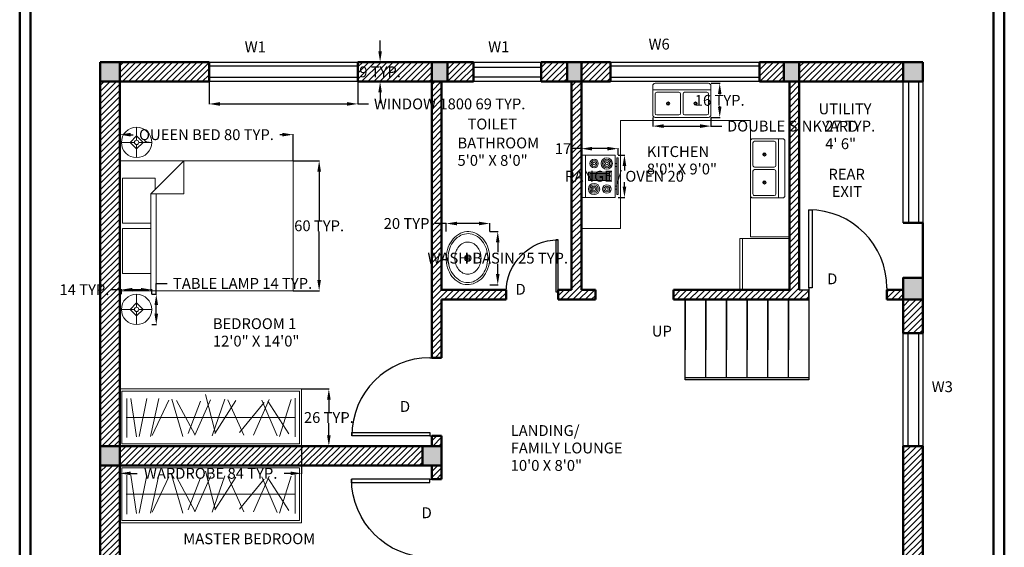
# Model space of a CAD drawing. Units: inches. Extents: x -25 to 429, y -18 to 847.
# Tile 2 of 3: x -25 to 429, y 226 to 470. Entities that reach past the tile are written whole.
import ezdxf

# ---------------------------------------------------------------- set-up
doc = ezdxf.new("R2010")
doc.units = ezdxf.units.IN
doc.header["$MEASUREMENT"] = 0
for name, color, linetype, lineweight in [('A-ANNO-DIMS', 2, 'Continuous', 18), ('A-ANNO-TEXT', 3, 'Continuous', 25), ('A-ANNO-TTLB', 7, 'Continuous', 50), ('A-AREA-IDEN', 7, 'Continuous', 25), ('A-DOOR', 4, 'Continuous', 25), ('A-FLOR-FIXT', 8, 'Continuous', 18), ('A-FLOR-STRS', 3, 'Continuous', 25), ('A-FURN', 8, 'Continuous', 18), ('A-GLAZ', 4, 'Continuous', 25), ('A-WALL', 7, 'Continuous', 50), ('A-WALL-FILL', 18, 'Continuous', 13), ('A-WALL-PATT', 252, 'Continuous', 13)]:
    doc.layers.add(name, color=color, linetype=linetype, lineweight=lineweight)
doc.styles.get("Standard").update_dxf_attribs({"font": 'arial.ttf'})
doc.dimstyles.get("Standard").update_dxf_attribs({"dimtxt": 5, "dimasz": 5, "dimexe": 0.18, "dimexo": 0.0625, "dimgap": 0.09, "dimtad": 0, "dimtih": 1, "dimtoh": 1, "dimdec": 1, "dimzin": 0, "dimdsep": 46, "dimlunit": 4, "dimtxsty": 'Standard', "dimcen": 0.09, "dimadec": 0, "dimazin": 0, "dimtfac": 1, "dimtdec": 1, "dimtofl": 0, "dimtmove": 0, "dimatfit": 3, "dimfxl": 1, "dimtolj": 1, "dimtzin": 0, "dimarcsym": 0})

# ---------------------------------------------------------------- blocks, each defined once
blk = doc.blocks.new('Bed - Queen')
for p, q in [((0, -80.00003), (0, 0)), ((0, 0), (59.99999, 0)), ((59.99999, 0), (59.99999, -80.00003)), ((7.99999, -1.2), (28.79998, -1.2)), ((7.99999, -14.4), (7.99999, -1.2)), ((28.79998, -1.2), (28.79998, -14.4)), ((31.19999, -1.2), (51.99999, -1.2)), ((31.19999, -14.4), (31.19999, -1.2)), ((51.99999, -1.2), (51.99999, -16.4)), ((0, -14.4), (44.8, -14.4)), ((44.8, -16.8), (0, -16.8)), ((59.99999, -29.6), (44.8, -14.4)), ((44.8, -14.4), (44.8, -29.6)), ((51.99999, -16.4), (46.79936, -16.4)), ((44.8, -29.6), (59.99999, -29.6)), ((59.99999, -80.00003), (0, -80.00003))]:
    blk.add_line(p, q)
blk = doc.blocks.new('Lamp - Table')
for p, q in [((0, 7), (0, 1)), ((-1, 0), (-7, 0)), ((0, 3), (-3, 0)), ((-3, 0), (0, -3)), ((3, 0), (0, 3)), ((0, -3), (3, 0)), ((1, 0), (7, 0)), ((0, -1), (0, -7))]:
    blk.add_line(p, q)
for radius in [7, 1]:
    blk.add_circle((0, 0), radius)
blk = doc.blocks.new('Range-Oven - 30 in top')
for p, q in [((0, -3), (30, -3)), ((12, -6), (18, -6)), ((13, -20), (13, -6)), ((14, -6), (14, -20)), ((15, -20), (15, -6)), ((16, -6), (16, -20)), ((17, -20), (17, -6)), ((18, -20), (12, -20)), ((6, -24), (6, -25)), ((8, -25), (8, -24)), ((22, -25), (22, -24)), ((24, -24), (24, -25))]:
    blk.add_line(p, q)
for points in [[(0, -24), (0, 0), (30, 0), (30, -24)], [(12, -21), (12, -5), (18, -5), (18, -21)], [(2, -26), (2, -25), (28, -25), (28, -26)]]:
    blk.add_lwpolyline(points, close=True)
for centre, radius in [((6, -9), 4), ((6, -9), 3), ((24, -9), 3), ((6, -9), 2), ((6, -9), 1), ((24, -9), 2), ((24, -9), 1), ((6, -18), 3), ((6, -18), 2), ((6, -18), 1), ((24, -18), 4), ((24, -18), 3), ((24, -18), 2), ((24, -18), 1)]:
    blk.add_circle(centre, radius)
blk = doc.blocks.new('Sink-double - 36 in top')
for p, q in [((-18, -4), (18, -4)), ((-0.75, -18.5), (-0.75, -6.5)), ((0.75, -6.5), (0.75, -18.5))]:
    blk.add_line(p, q)
for points in [[(-16.5, 0), (16.5, 0)], [(-18, -19.5), (-18, -1.5)], [(-15.5, -5.5), (-1.75, -5.5)], [(1.75, -5.5), (15.5, -5.5)], [(18, -1.5), (18, -19.5)], [(-16.5, -18.5), (-16.5, -6.5)], [(16.5, -6.5), (16.5, -18.5)], [(16.5, -21), (-16.5, -21)], [(-1.75, -19.5), (-15.5, -19.5)], [(15.5, -19.5), (1.75, -19.5)]]:
    blk.add_lwpolyline(points)
for centre, radius in [((-8.5, -12.5), 1), ((8.5, -12.5), 1), ((-8.5, -12.5), 0.5), ((8.5, -12.5), 0.5)]:
    blk.add_circle(centre, radius)
for centre, radius, start, end in [((-16.5, -1.5), 1.5, 90, 180), ((16.5, -1.5), 1.5, 0, 90), ((-15.5, -6.5), 1, 90, 180), ((-1.75, -6.5), 1, 0, 90), ((1.75, -6.5), 1, 90, 180), ((15.5, -6.5), 1, 0, 90), ((-16.5, -19.5), 1.5, 180, 270), ((-15.5, -18.5), 1, 180, 270), ((-1.75, -18.5), 1, 270, 0), ((1.75, -18.5), 1, 180, 270), ((15.5, -18.5), 1, 270, 0), ((16.5, -19.5), 1.5, 270, 0)]:
    blk.add_arc(centre, radius, start, end)
blk = doc.blocks.new('Sink - Oval top')
for p, q in [((-1, 0), (1, 0)), ((0, 1), (0, -1))]:
    blk.add_line(p, q)
for points in [[(-12.23, 0.39, 0.117634), (-11.46, -3.36, 0.104469), (-8.88, -6.8, 0.090016), (-5.08, -9.07, 0.08192), (-0.32, -10.02, 0.08192), (4.49, -9.38, 0.090016), (8.42, -7.36, 0.104469), (11.22, -4.09, 0.117634), (12.23, -0.39, 0.117634), (11.46, 3.36, 0.104469), (8.88, 6.8, 0.090016), (5.08, 9.07, 0.08192), (0.32, 10.02, 0.08192), (-4.49, 9.38, 0.090016), (-8.42, 7.36, 0.104469), (-11.22, 4.09, 0.117634)], [(-11.29, 0.16, 0.118622), (-10.52, -3.25, 0.104678), (-8.07, -6.36, 0.089562), (-4.54, -8.37, 0.081185), (-0.13, -9.15, 0.081185), (4.3, -8.49, 0.089562), (7.89, -6.58, 0.104678), (10.42, -3.55, 0.118622), (11.29, -0.16, 0.118622), (10.52, 3.25, 0.104678), (8.07, 6.36, 0.089562), (4.54, 8.37, 0.081185), (0.13, 9.15, 0.081185), (-4.3, 8.49, 0.089562), (-7.89, 6.58, 0.104678), (-10.42, 3.55, 0.118622)], [(-7.42, 0.08, 0.118283), (-6.91, -2.17, 0.104607), (-5.29, -4.21, 0.089718), (-2.97, -5.53, 0.081436), (-0.07, -6.04, 0.081436), (2.84, -5.59, 0.089718), (5.2, -4.33, 0.104607), (6.86, -2.32, 0.118283), (7.42, -0.08, 0.118283), (6.91, 2.17, 0.104607), (5.29, 4.21, 0.089718), (2.97, 5.53, 0.081436), (0.07, 6.04, 0.081436), (-2.84, 5.59, 0.089718), (-5.2, 4.33, 0.104607), (-6.86, 2.32, 0.118283)]]:
    blk.add_lwpolyline(points, format="xyb", close=True)
for radius in [1.5, 1]:
    blk.add_circle((0, 0), radius)
blk = doc.blocks.new('*U10')
for p, q in [((0, 0), (0, -6)), ((40, 0), (40, -6))]:
    blk.add_line(p, q)
blk.add_lwpolyline([(0, 0), (0, 40), (1.75, 40), (1.75, 0)], close=True)
blk.add_arc((0, 0), 40, 0, 90)
blk = doc.blocks.new('WIN-1800')
for points in [[(62.34, 449.99), (130.96, 449.99), (130.96, 440.99), (62.34, 440.99)], [(62.34, 448.22), (130.96, 448.22), (130.96, 442.88), (62.34, 442.88)]]:
    blk.add_lwpolyline(points, close=True)
blk = doc.blocks.new('WARDROBE')
for p, q in [((65.2, 279.42), (60.7, 296.77)), ((24.4, 294.9), (24.4, 276.98)), ((26.21, 294.93), (28.79, 277.19)), ((30.1, 277.36), (33.56, 294.94)), ((35.31, 277.4), (39.12, 294.91)), ((43.72, 294.1), (36.12, 277.87)), ((50.25, 277.42), (45.12, 294.59)), ((55.73, 278.26), (47.25, 294.05)), ((52.63, 278.85), (58.34, 293.66)), ((63.03, 294.35), (55.8, 277.95)), ((69.66, 294.66), (63.69, 277.76)), ((74.73, 293.93), (65.06, 278.84)), ((71.01, 294.33), (78.36, 277.98)), ((76.36, 279.22), (87.72, 293.08)), ((82.89, 277.99), (90.13, 294.39)), ((86.74, 294.18), (93.8, 277.71)), ((99.06, 278.61), (89.44, 293.73)), ((100.23, 294.49), (94.82, 277.41)), ((102.02, 277.19), (102.02, 295.11)), ((24.13, 286.15), (102.02, 286.15)), ((87.63, 286.15), (69.71, 286.15))]:
    blk.add_line(p, q)
for points in [[(21.13, 272.99), (105.02, 272.99), (105.02, 299.31), (21.13, 299.31)], [(22.13, 273.99), (104.02, 273.99), (104.02, 298.31), (22.13, 298.31)]]:
    blk.add_lwpolyline(points, close=True)
blk = doc.blocks.new('*D13')
at = {"layer": 'A-ANNO-DIMS', "color": 0, "lineweight": -2, "ltscale": 0.5, "transparency": 16777216}
for p, q in [((37.97, 342.96), (37.97, 347.96)), ((37.97, 347.96), (42.97, 347.96)), ((35.93, 342.96), (38.15, 342.96)), ((37.97, 333.96), (37.97, 337.96)), ((35.93, 328.96), (38.15, 328.96))]:
    blk.add_line(p, q, dxfattribs=at)
at = {"layer": 'A-ANNO-DIMS', "color": 0, "lineweight": 100, "ltscale": 0.5, "transparency": 16777216}
for points in [[(37.13, 337.96), (38.8, 337.96), (37.97, 342.96)], [(37.13, 333.96), (38.8, 333.96), (37.97, 328.96)]]:
    blk.add_solid(points, dxfattribs=at)
at = {"layer": 'Defpoints', "color": 0, "lineweight": 100, "ltscale": 0.5, "transparency": 16777216}
for p in [(35.87, 342.96), (37.97, 342.96), (35.87, 328.96)]:
    blk.add_point(p, dxfattribs=at)
at = {"layer": 'A-ANNO-DIMS', "color": 0, "ltscale": 0.5, "transparency": 16777216, "insert": (77.8, 347.96), "char_height": 5, "attachment_point": 5}
blk.add_mtext('\\A1;TABLE LAMP 14 TYP.', dxfattribs=at)
blk = doc.blocks.new('*D14')
at = {"layer": 'A-ANNO-DIMS', "color": 0, "lineweight": -2, "ltscale": 0.5, "transparency": 16777216}
for p, q in [((21.87, 345.06), (16.87, 345.06)), ((21.87, 343.02), (21.87, 345.24)), ((30.87, 345.06), (26.87, 345.06)), ((35.87, 343.02), (35.87, 345.24))]:
    blk.add_line(p, q, dxfattribs=at)
at = {"layer": 'A-ANNO-DIMS', "color": 0, "lineweight": 100, "ltscale": 0.5, "transparency": 16777216}
for points in [[(26.87, 345.89), (26.87, 344.23), (21.87, 345.06)], [(30.87, 345.89), (30.87, 344.23), (35.87, 345.06)]]:
    blk.add_solid(points, dxfattribs=at)
at = {"layer": 'Defpoints', "color": 0, "lineweight": 100, "ltscale": 0.5, "transparency": 16777216}
for p in [(21.87, 345.06), (21.87, 342.96), (35.87, 342.96)]:
    blk.add_point(p, dxfattribs=at)
at = {"layer": 'A-ANNO-DIMS', "color": 0, "ltscale": 0.5, "transparency": 16777216, "insert": (4.84, 345.06), "char_height": 5, "attachment_point": 5}
blk.add_mtext('\\A1;14 TYP.', dxfattribs=at)
blk = doc.blocks.new('*D15')
at = {"layer": 'A-ANNO-DIMS', "color": 0, "lineweight": -2, "ltscale": 0.5, "transparency": 16777216}
for p, q in [((191.92, 371.9), (195.72, 371.9)), ((195.54, 366.9), (195.54, 362.3)), ((195.54, 352.35), (195.54, 356.95)), ((191.92, 347.35), (195.72, 347.35))]:
    blk.add_line(p, q, dxfattribs=at)
at = {"layer": 'A-ANNO-DIMS', "color": 0, "lineweight": 100, "ltscale": 0.5, "transparency": 16777216}
for points in [[(194.7, 366.9), (196.37, 366.9), (195.54, 371.9)], [(194.7, 352.35), (196.37, 352.35), (195.54, 347.35)]]:
    blk.add_solid(points, dxfattribs=at)
at = {"layer": 'Defpoints', "color": 0, "lineweight": 100, "ltscale": 0.5, "transparency": 16777216}
for p in [(191.85, 371.9), (195.54, 371.9), (191.85, 347.35)]:
    blk.add_point(p, dxfattribs=at)
at = {"layer": 'A-ANNO-DIMS', "color": 0, "ltscale": 0.5, "transparency": 16777216, "insert": (195.54, 359.62), "char_height": 5, "attachment_point": 5}
blk.add_mtext('\\A1;WASH BASIN 25 TYP.', dxfattribs=at)
blk = doc.blocks.new('*D16')
at = {"layer": 'A-ANNO-DIMS', "color": 0, "lineweight": -2, "ltscale": 0.5, "transparency": 16777216}
for p, q in [((171.72, 375.58), (166.72, 375.58)), ((171.72, 371.96), (171.72, 375.76)), ((186.85, 375.58), (176.72, 375.58)), ((191.85, 371.96), (191.85, 375.76))]:
    blk.add_line(p, q, dxfattribs=at)
at = {"layer": 'A-ANNO-DIMS', "color": 0, "lineweight": 100, "ltscale": 0.5, "transparency": 16777216}
for points in [[(176.72, 376.41), (176.72, 374.75), (171.72, 375.58)], [(186.85, 376.41), (186.85, 374.75), (191.85, 375.58)]]:
    blk.add_solid(points, dxfattribs=at)
at = {"layer": 'Defpoints', "color": 0, "lineweight": 100, "ltscale": 0.5, "transparency": 16777216}
for p in [(171.72, 375.58), (171.72, 371.9), (191.85, 371.9)]:
    blk.add_point(p, dxfattribs=at)
at = {"layer": 'A-ANNO-DIMS', "color": 0, "ltscale": 0.5, "transparency": 16777216, "insert": (154.41, 375.58), "char_height": 5, "attachment_point": 5}
blk.add_mtext('\\A1;20 TYP.', dxfattribs=at)
blk = doc.blocks.new('*D17')
at = {"layer": 'A-ANNO-DIMS', "color": 0, "lineweight": -2, "ltscale": 0.5, "transparency": 16777216}
for p, q in [((21.13, 404.6), (21.13, 416.71)), ((26.13, 416.53), (27.33, 416.53)), ((96.13, 416.53), (94.92, 416.53)), ((101.13, 404.6), (101.13, 416.71))]:
    blk.add_line(p, q, dxfattribs=at)
at = {"layer": 'A-ANNO-DIMS', "color": 0, "lineweight": 100, "ltscale": 0.5, "transparency": 16777216}
for points in [[(26.13, 417.37), (26.13, 415.7), (21.13, 416.53)], [(96.13, 417.37), (96.13, 415.7), (101.13, 416.53)]]:
    blk.add_solid(points, dxfattribs=at)
at = {"layer": 'Defpoints', "color": 0, "lineweight": 100, "ltscale": 0.5, "transparency": 16777216}
for p in [(21.13, 416.53), (21.13, 404.53), (101.13, 404.53)]:
    blk.add_point(p, dxfattribs=at)
at = {"layer": 'A-ANNO-DIMS', "color": 0, "ltscale": 0.5, "transparency": 16777216, "insert": (61.13, 416.53), "char_height": 5, "attachment_point": 5}
blk.add_mtext('\\A1;QUEEN BED 80 TYP.', dxfattribs=at)
blk = doc.blocks.new('*D18')
at = {"layer": 'A-ANNO-DIMS', "color": 0, "lineweight": -2, "ltscale": 0.5, "transparency": 16777216}
for p, q in [((101.19, 404.53), (113.31, 404.53)), ((113.13, 399.53), (113.13, 377.18)), ((113.13, 349.53), (113.13, 371.89)), ((101.19, 344.53), (113.31, 344.53))]:
    blk.add_line(p, q, dxfattribs=at)
at = {"layer": 'A-ANNO-DIMS', "color": 0, "lineweight": 100, "ltscale": 0.5, "transparency": 16777216}
for points in [[(112.29, 399.53), (113.96, 399.53), (113.13, 404.53)], [(112.29, 349.53), (113.96, 349.53), (113.13, 344.53)]]:
    blk.add_solid(points, dxfattribs=at)
at = {"layer": 'Defpoints', "color": 0, "lineweight": 100, "ltscale": 0.5, "transparency": 16777216}
for p in [(101.13, 404.53), (113.13, 404.53), (101.13, 344.53)]:
    blk.add_point(p, dxfattribs=at)
at = {"layer": 'A-ANNO-DIMS', "color": 0, "ltscale": 0.5, "transparency": 16777216, "insert": (113.13, 374.53), "char_height": 5, "attachment_point": 5}
blk.add_mtext('\\A1;60 TYP.', dxfattribs=at)
blk = doc.blocks.new('*D27')
at = {"layer": 'A-ANNO-DIMS', "color": 0, "lineweight": -2, "ltscale": 0.5, "transparency": 16777216}
for p, q in [((267.02, 424.45), (267.02, 420.3)), ((293.92, 424.45), (293.92, 420.3)), ((272.02, 420.48), (288.92, 420.48)), ((293.92, 420.48), (298.92, 420.48))]:
    blk.add_line(p, q, dxfattribs=at)
at = {"layer": 'A-ANNO-DIMS', "color": 0, "lineweight": 100, "ltscale": 0.5, "transparency": 16777216}
for points in [[(272.02, 421.31), (272.02, 419.65), (267.02, 420.48)], [(288.92, 421.31), (288.92, 419.65), (293.92, 420.48)]]:
    blk.add_solid(points, dxfattribs=at)
at = {"layer": 'Defpoints', "color": 0, "lineweight": 100, "ltscale": 0.5, "transparency": 16777216}
for p in [(267.02, 424.51), (293.92, 424.51), (293.92, 420.48)]:
    blk.add_point(p, dxfattribs=at)
at = {"layer": 'A-ANNO-DIMS', "color": 0, "ltscale": 0.5, "transparency": 16777216, "insert": (335.5, 420.48), "char_height": 5, "attachment_point": 5}
blk.add_mtext('\\A1;DOUBLE SINK 27 TYP.', dxfattribs=at)
blk = doc.blocks.new('*D28')
at = {"layer": 'A-ANNO-DIMS', "color": 0, "lineweight": -2, "ltscale": 0.5, "transparency": 16777216}
for p, q in [((293.98, 440.21), (298.13, 440.21)), ((297.95, 435.21), (297.95, 435)), ((297.95, 429.51), (297.95, 429.72)), ((293.98, 424.51), (298.13, 424.51))]:
    blk.add_line(p, q, dxfattribs=at)
at = {"layer": 'A-ANNO-DIMS', "color": 0, "lineweight": 100, "ltscale": 0.5, "transparency": 16777216}
for points in [[(297.12, 435.21), (298.78, 435.21), (297.95, 440.21)], [(297.12, 429.51), (298.78, 429.51), (297.95, 424.51)]]:
    blk.add_solid(points, dxfattribs=at)
at = {"layer": 'Defpoints', "color": 0, "lineweight": 100, "ltscale": 0.5, "transparency": 16777216}
for p in [(293.92, 440.21), (297.95, 440.21), (293.92, 424.51)]:
    blk.add_point(p, dxfattribs=at)
at = {"layer": 'A-ANNO-DIMS', "color": 0, "ltscale": 0.5, "transparency": 16777216, "insert": (297.95, 432.36), "char_height": 5, "attachment_point": 5}
blk.add_mtext('\\A1;16 TYP.', dxfattribs=at)
blk = doc.blocks.new('*D29')
at = {"layer": 'A-ANNO-DIMS', "color": 0, "lineweight": -2, "ltscale": 0.5, "transparency": 16777216}
for p, q in [((62.34, 440.93), (62.34, 430.52)), ((130.96, 440.93), (130.96, 430.52)), ((67.34, 430.7), (125.96, 430.7)), ((130.96, 430.7), (135.96, 430.7))]:
    blk.add_line(p, q, dxfattribs=at)
at = {"layer": 'A-ANNO-DIMS', "color": 0, "lineweight": 100, "ltscale": 0.5, "transparency": 16777216}
for points in [[(67.34, 431.53), (67.34, 429.86), (62.34, 430.7)], [(125.96, 431.53), (125.96, 429.86), (130.96, 430.7)]]:
    blk.add_solid(points, dxfattribs=at)
at = {"layer": 'Defpoints', "color": 0, "lineweight": 100, "ltscale": 0.5, "transparency": 16777216}
for p in [(62.34, 440.99), (130.96, 440.99), (130.96, 430.7)]:
    blk.add_point(p, dxfattribs=at)
at = {"layer": 'A-ANNO-DIMS', "color": 0, "ltscale": 0.5, "transparency": 16777216, "insert": (173.35, 430.7), "char_height": 5, "attachment_point": 5}
blk.add_mtext('\\A1;WINDOW 1800 69 TYP.', dxfattribs=at)
blk = doc.blocks.new('*D30')
at = {"layer": 'A-ANNO-DIMS', "color": 0, "lineweight": -2, "ltscale": 0.5, "transparency": 16777216}
for p, q in [((141.25, 454.99), (141.25, 459.99)), ((131.02, 449.99), (141.43, 449.99)), ((131.02, 440.99), (141.43, 440.99)), ((141.25, 435.99), (141.25, 430.99))]:
    blk.add_line(p, q, dxfattribs=at)
at = {"layer": 'A-ANNO-DIMS', "color": 0, "lineweight": 100, "ltscale": 0.5, "transparency": 16777216}
for points in [[(140.42, 454.99), (142.09, 454.99), (141.25, 449.99)], [(140.42, 435.99), (142.09, 435.99), (141.25, 440.99)]]:
    blk.add_solid(points, dxfattribs=at)
at = {"layer": 'Defpoints', "color": 0, "lineweight": 100, "ltscale": 0.5, "transparency": 16777216}
for p in [(130.96, 449.99), (141.25, 449.99), (130.96, 440.99)]:
    blk.add_point(p, dxfattribs=at)
at = {"layer": 'A-ANNO-DIMS', "color": 0, "ltscale": 0.5, "transparency": 16777216, "insert": (141.25, 445.49), "char_height": 5, "attachment_point": 5}
blk.add_mtext('\\A1;9 TYP.', dxfattribs=at)
blk = doc.blocks.new('*D31')
at = {"layer": 'A-ANNO-DIMS', "color": 0, "lineweight": -2, "ltscale": 0.5, "transparency": 16777216}
for p, q in [((21.13, 272.93), (21.13, 260.23)), ((105.02, 272.93), (105.02, 260.23)), ((26.13, 260.41), (29.17, 260.41)), ((100.02, 260.41), (96.97, 260.41))]:
    blk.add_line(p, q, dxfattribs=at)
at = {"layer": 'A-ANNO-DIMS', "color": 0, "lineweight": 100, "ltscale": 0.5, "transparency": 16777216}
for points in [[(26.13, 261.24), (26.13, 259.57), (21.13, 260.41)], [(100.02, 261.24), (100.02, 259.57), (105.02, 260.41)]]:
    blk.add_solid(points, dxfattribs=at)
at = {"layer": 'Defpoints', "color": 0, "lineweight": 100, "ltscale": 0.5, "transparency": 16777216}
for p in [(21.13, 272.99), (105.02, 272.99), (105.02, 260.41)]:
    blk.add_point(p, dxfattribs=at)
at = {"layer": 'A-ANNO-DIMS', "color": 0, "ltscale": 0.5, "transparency": 16777216, "insert": (63.07, 260.41), "char_height": 5, "attachment_point": 5}
blk.add_mtext('\\A1;WARDROBE 84 TYP.', dxfattribs=at)
blk = doc.blocks.new('*D32')
at = {"layer": 'A-ANNO-DIMS', "color": 0, "lineweight": -2, "ltscale": 0.5, "transparency": 16777216}
for p, q in [((105.08, 299.31), (117.78, 299.31)), ((117.6, 294.31), (117.6, 288.79)), ((117.6, 277.99), (117.6, 283.51)), ((105.08, 272.99), (117.78, 272.99))]:
    blk.add_line(p, q, dxfattribs=at)
at = {"layer": 'A-ANNO-DIMS', "color": 0, "lineweight": 100, "ltscale": 0.5, "transparency": 16777216}
for points in [[(116.77, 294.31), (118.44, 294.31), (117.6, 299.31)], [(116.77, 277.99), (118.44, 277.99), (117.6, 272.99)]]:
    blk.add_solid(points, dxfattribs=at)
at = {"layer": 'Defpoints', "color": 0, "lineweight": 100, "ltscale": 0.5, "transparency": 16777216}
for p in [(105.02, 299.31), (117.6, 299.31), (105.02, 272.99)]:
    blk.add_point(p, dxfattribs=at)
at = {"layer": 'A-ANNO-DIMS', "color": 0, "ltscale": 0.5, "transparency": 16777216, "insert": (117.6, 286.15), "char_height": 5, "attachment_point": 5}
blk.add_mtext('\\A1;26 TYP.', dxfattribs=at)
blk = doc.blocks.new('*D33')
at = {"layer": 'A-ANNO-DIMS', "color": 0, "lineweight": -2, "ltscale": 0.5, "transparency": 16777216}
for p, q in [((251.13, 407.15), (254.18, 407.15)), ((254, 402.15), (254, 400.04)), ((254, 392.57), (254, 394.68)), ((251.13, 387.57), (254.18, 387.57))]:
    blk.add_line(p, q, dxfattribs=at)
at = {"layer": 'A-ANNO-DIMS', "color": 0, "lineweight": 100, "ltscale": 0.5, "transparency": 16777216}
for points in [[(253.17, 402.15), (254.84, 402.15), (254, 407.15)], [(253.17, 392.57), (254.84, 392.57), (254, 387.57)]]:
    blk.add_solid(points, dxfattribs=at)
at = {"layer": 'Defpoints', "color": 0, "lineweight": 100, "ltscale": 0.5, "transparency": 16777216}
for p in [(251.07, 407.15), (254, 407.15), (251.07, 387.57)]:
    blk.add_point(p, dxfattribs=at)
at = {"layer": 'A-ANNO-DIMS', "color": 0, "ltscale": 0.5, "transparency": 16777216, "insert": (254, 397.36), "char_height": 5, "attachment_point": 5}
blk.add_mtext('\\A1;RANGE / OVEN 20', dxfattribs=at)
blk = doc.blocks.new('*D34')
at = {"layer": 'A-ANNO-DIMS', "color": 0, "lineweight": -2, "ltscale": 0.5, "transparency": 16777216}
for p, q in [((234.1, 410.08), (229.1, 410.08)), ((234.1, 407.21), (234.1, 410.26)), ((246.07, 410.08), (239.1, 410.08)), ((251.07, 407.21), (251.07, 410.26))]:
    blk.add_line(p, q, dxfattribs=at)
at = {"layer": 'A-ANNO-DIMS', "color": 0, "lineweight": 100, "ltscale": 0.5, "transparency": 16777216}
for points in [[(239.1, 410.92), (239.1, 409.25), (234.1, 410.08)], [(246.07, 410.92), (246.07, 409.25), (251.07, 410.08)]]:
    blk.add_solid(points, dxfattribs=at)
at = {"layer": 'Defpoints', "color": 0, "lineweight": 100, "ltscale": 0.5, "transparency": 16777216}
for p in [(234.1, 410.08), (234.1, 407.15), (251.07, 407.15)]:
    blk.add_point(p, dxfattribs=at)
at = {"layer": 'A-ANNO-DIMS', "color": 0, "ltscale": 0.5, "transparency": 16777216, "insert": (225.67, 410.08), "char_height": 5, "attachment_point": 5}
blk.add_mtext('\\A1;17', dxfattribs=at)

msp = doc.modelspace()

# ---------------------------------------------------------------- hatches: boundary and pattern name
at = {"layer": 'A-WALL-FILL'}
h = msp.add_hatch(color=256, dxfattribs=at)
h.dxf.hatch_style = 1
h.paths.add_polyline_path([(169.63, 272.99), (160.88, 272.99), (160.88, 263.99), (169.63, 263.99)])
h.paths.add_polyline_path([(21.13, 95.99), (12.13, 95.99), (12.13, 86.99), (21.13, 86.99)])
h.paths.add_polyline_path([(21.13, 272.99), (12.13, 272.99), (12.13, 263.99), (21.13, 263.99)])
h.paths.add_polyline_path([(391.63, 350.55), (382.63, 350.55), (382.63, 340.49), (391.63, 340.49)])
h.paths.add_polyline_path([(391.63, 71.99), (382.63, 71.99), (382.63, 62.99), (391.63, 62.99)])
h.paths.add_polyline_path([(391.63, 220.21), (382.63, 220.21), (382.63, 208.25), (391.63, 208.25)])
h.paths.add_polyline_path([(334.63, 449.99), (327.59, 449.99), (327.59, 440.99), (334.63, 440.99)])
h.paths.add_polyline_path([(391.63, 449.99), (382.63, 449.99), (382.63, 440.99), (391.63, 440.99)])
h.paths.add_polyline_path([(234.13, 449.99), (227.53, 449.99), (227.53, 440.99), (234.13, 440.99)])
h.paths.add_polyline_path([(172.34, 449.99), (165.13, 449.99), (165.13, 440.99), (172.34, 440.99)])
h.paths.add_polyline_path([(21.13, 449.99), (12.13, 449.99), (12.13, 440.99), (21.13, 440.99)])
at = {"layer": 'A-WALL-PATT'}
h = msp.add_hatch(dxfattribs=at)
h.set_pattern_fill('ANSI31', color=256, scale=16)
h.paths.add_polyline_path([(160.88, 272.99), (21.13, 272.99), (21.13, 263.99), (105.02, 263.99), (160.88, 263.99)])
h.paths.add_polyline_path([(169.63, 340.49), (199.38, 340.49), (199.38, 344.99), (169.63, 344.99), (169.63, 440.99), (165.13, 440.99), (165.13, 313.72), (169.63, 313.72)])
h.paths.add_polyline_path([(21.13, 440.99), (12.13, 440.99), (12.13, 272.99), (21.13, 272.99), (21.13, 299.31)])
h.paths.add_polyline_path([(62.34, 449.99), (21.13, 449.99), (21.13, 440.99), (62.34, 440.99)])
h.paths.add_polyline_path([(165.13, 449.99), (130.96, 449.99), (130.96, 440.99), (165.13, 440.99)])
h.paths.add_polyline_path([(184.34, 449.99), (172.34, 449.99), (172.34, 440.99), (184.34, 440.99)])
h.paths.add_polyline_path([(227.53, 449.99), (215.51, 449.99), (215.51, 440.99), (227.53, 440.99)])
h.paths.add_polyline_path([(247.61, 449.99), (234.13, 449.99), (234.13, 440.99), (247.61, 440.99)])
h.paths.add_polyline_path([(327.59, 449.99), (316.24, 449.99), (316.24, 440.99), (327.59, 440.99)])
h.paths.add_polyline_path([(234.1, 407.15), (234.12, 440.99), (229.63, 440.99), (229.63, 344.99), (223.38, 344.99), (223.38, 340.49), (240.63, 340.49), (240.63, 344.99), (234.13, 344.99), (234.13, 387.57), (234.1, 387.57)])
h.paths.add_polyline_path([(334.63, 440.99), (330.13, 440.99), (330.13, 344.99), (276.63, 344.99), (276.63, 340.49), (339.1, 340.49), (339.1, 344.99), (334.63, 344.99)])
h.paths.add_polyline_path([(382.63, 449.99), (334.63, 449.99), (334.63, 440.99), (382.63, 440.99)])
h.paths.add_polyline_path([(382.63, 344.99), (375.1, 344.99), (375.1, 340.49), (382.63, 340.49)])
h.paths.add_polyline_path([(391.63, 340.49), (382.63, 340.49), (382.63, 325.05), (391.63, 325.05)])
h.paths.add_polyline_path([(391.63, 273.01), (382.63, 273.01), (382.63, 220.21), (391.63, 220.21)])
h.paths.add_polyline_path([(391.63, 208.25), (382.63, 208.25), (382.63, 71.99), (391.63, 71.99)])
h.paths.add_polyline_path([(382.63, 71.99), (330.34, 71.99), (330.34, 62.99), (382.63, 62.99)])
h.paths.add_polyline_path([(262.4, 71.99), (235.63, 71.99), (235.63, 208.49), (224.79, 208.49), (224.79, 203.99), (231.13, 203.99), (231.13, 95.99), (169.63, 95.99), (169.63, 203.99), (200.79, 203.99), (200.79, 208.49), (169.63, 208.49), (169.63, 221.76), (165.13, 221.76), (165.13, 95.99), (154.17, 95.99), (154.17, 86.99), (231.13, 86.99), (231.13, 62.99), (262.4, 62.99)])
h.paths.add_polyline_path([(48.08, 95.99), (21.13, 95.99), (21.13, 86.99), (48.08, 86.99)])
h.paths.add_polyline_path([(21.13, 263.99), (12.13, 263.99), (12.13, 95.99), (21.13, 95.99)])
h.paths.add_polyline_path([(169.63, 263.99), (165.13, 263.99), (165.13, 257.76), (169.63, 257.76)])
h.paths.add_polyline_path([(169.63, 277.72), (165.13, 277.72), (165.13, 272.99), (169.63, 272.99)])

# ---------------------------------------------------------------- linework, layer by layer
at = {"layer": 'A-ANNO-TTLB', "ltscale": 0.5}
for points in [[(-25.05, 846.91), (429.28, 846.91), (429.28, -17.53), (-25.05, -17.53)], [(-20.05, 841.91), (424.28, 841.91), (424.28, -12.53), (-20.05, -12.53)]]:
    msp.add_lwpolyline(points, close=True, dxfattribs=at)
at = {"layer": 'A-FLOR-FIXT'}
for p, q in [((252.13, 373.32), (252.13, 422.99)), ((252.13, 422.99), (312.13, 422.99)), ((312.13, 422.99), (312.13, 369.49)), ((234.13, 373.32), (252.13, 373.32)), ((308.45, 368.71), (308.41, 345.02)), ((312.13, 369.49), (330.13, 369.49)), ((312.13, 345.02), (312.13, 344.99))]:
    msp.add_line(p, q, dxfattribs=at)
msp.add_lwpolyline([(330.13, 344.99), (307.3, 345.03), (307.3, 368.71), (330.13, 368.67)], close=True, dxfattribs=at)
at = {"layer": 'A-FLOR-STRS'}
for p, q in [((334.63, 344.99), (339.1, 344.99)), ((339.1, 340.49), (339.1, 344.99)), ((281.95, 303.49), (281.95, 340.49)), ((281.95, 340.49), (281.95, 317.33)), ((291.49, 304.49), (291.49, 340.49)), ((291.49, 340.49), (291.49, 317.33)), ((301.02, 304.49), (301.02, 340.49)), ((301.02, 340.49), (301.02, 317.33)), ((310.56, 304.49), (310.56, 340.49)), ((310.56, 340.49), (310.56, 317.33)), ((320.1, 304.49), (320.1, 340.49)), ((320.1, 340.49), (320.1, 317.33)), ((329.63, 304.49), (329.63, 340.49)), ((329.63, 340.49), (329.63, 317.33)), ((339.1, 340.49), (339.1, 303.49)), ((339.1, 304.49), (281.95, 304.49)), ((339.1, 303.49), (281.95, 303.49))]:
    msp.add_line(p, q, dxfattribs=at)
at = {"layer": 'A-GLAZ'}
for points in [[(184.34, 449.99), (215.51, 449.99), (215.51, 440.99), (184.34, 440.99)], [(184.34, 447.66), (215.51, 447.66), (215.51, 443.03), (184.34, 443.03)], [(382.63, 440.99), (391.63, 440.99), (391.63, 375.94), (382.63, 375.94)], [(385.24, 440.99), (389.64, 440.99), (389.64, 375.94), (385.24, 375.94)], [(382.63, 325.05), (391.63, 325.05), (391.63, 273.01), (382.63, 273.01)], [(384.98, 325.05), (389.63, 325.05), (389.63, 273.01), (384.98, 273.01)]]:
    msp.add_lwpolyline(points, close=True, dxfattribs=at)
at = {"layer": 'A-WALL'}
for p, q in [((12.13, 449.99), (62.34, 449.99)), ((12.13, 449.99), (12.13, 86.99)), ((21.13, 449.99), (21.13, 86.99)), ((62.34, 449.99), (62.34, 440.99)), ((130.96, 449.99), (130.96, 440.99)), ((130.96, 449.99), (184.34, 449.99)), ((165.13, 449.99), (165.13, 313.72)), ((184.34, 440.99), (184.34, 449.99)), ((215.51, 440.99), (215.51, 449.99)), ((215.51, 449.99), (247.61, 449.99)), ((234.13, 449.99), (234.13, 344.99)), ((247.61, 440.99), (247.61, 449.99)), ((316.24, 440.99), (316.24, 449.99)), ((316.24, 449.99), (391.63, 449.99)), ((334.63, 449.99), (334.63, 344.99)), ((382.63, 449.99), (382.63, 440.99)), ((391.63, 449.99), (391.63, 440.99)), ((12.13, 440.99), (62.34, 440.99)), ((130.96, 440.99), (165.13, 440.99)), ((169.63, 440.99), (169.63, 344.99)), ((169.63, 440.99), (184.34, 440.99)), ((215.51, 440.99), (229.63, 440.99)), ((229.63, 440.99), (229.63, 344.99)), ((234.13, 440.99), (247.61, 440.99)), ((316.24, 440.99), (391.63, 440.99)), ((330.13, 440.99), (330.13, 344.99)), ((382.63, 375.94), (391.63, 375.94)), ((382.63, 350.55), (382.63, 344.99)), ((391.63, 350.55), (391.63, 325.05)), ((169.63, 344.99), (199.38, 344.99)), ((199.38, 344.99), (199.38, 340.49)), ((223.38, 340.49), (223.38, 344.99)), ((223.38, 344.99), (229.63, 344.99)), ((234.13, 344.99), (240.63, 344.99)), ((240.63, 340.49), (240.63, 344.99)), ((276.63, 344.99), (276.63, 340.49)), ((276.63, 344.99), (330.13, 344.99)), ((375.1, 344.99), (375.1, 340.49)), ((375.1, 344.99), (382.63, 344.99)), ((169.63, 340.49), (199.38, 340.49)), ((169.63, 340.49), (169.63, 313.72)), ((223.38, 340.49), (240.63, 340.49)), ((276.63, 340.49), (339.1, 340.49)), ((375.1, 340.49), (382.63, 340.49)), ((382.63, 340.49), (382.63, 325.05)), ((382.63, 325.05), (391.63, 325.05)), ((165.13, 313.72), (169.63, 313.72)), ((169.63, 277.72), (165.13, 277.72)), ((165.13, 277.72), (165.13, 272.99)), ((169.63, 277.72), (169.63, 263.99)), ((12.13, 272.99), (165.13, 272.99)), ((382.63, 273.01), (391.63, 273.01)), ((382.63, 273.01), (382.63, 62.99)), ((391.63, 273.01), (391.63, 62.99)), ((12.13, 263.99), (165.13, 263.99)), ((165.13, 263.99), (165.13, 257.76)), ((169.63, 263.99), (169.63, 257.76)), ((169.63, 257.76), (165.13, 257.76))]:
    msp.add_line(p, q, dxfattribs=at)
at = {"layer": 'A-WALL', "ltscale": 0.2}
msp.add_line((391.63, 375.94), (391.63, 350.55), dxfattribs=at)
at = {"layer": 'A-WALL'}
for points in [[(165.13, 440.99), (172.34, 440.99), (172.34, 449.99), (165.13, 449.99)], [(234.13, 440.99), (227.53, 440.99), (227.53, 449.99), (234.13, 449.99)], [(334.63, 440.99), (327.59, 440.99), (327.59, 449.99), (334.63, 449.99)], [(382.63, 340.49), (391.63, 340.49), (391.63, 350.55), (382.63, 350.55)], [(169.63, 263.99), (160.88, 263.99), (160.88, 272.99), (169.63, 272.99)]]:
    msp.add_lwpolyline(points, close=True, dxfattribs=at)

# ---------------------------------------------------------------- block references
at = {"layer": 'A-DOOR'}
for p, xscale, yscale, zscale in [((339.1, 345.89), 0.8997003436788849, 0.8997003436788849, 0.8997003436788849), ((223.38, 344.09), -0.5992845134572276, 0.5992845134572276, 0.5992845134572276)]:
    msp.add_blockref('*U10', p, dxfattribs=dict(at, xscale=xscale, yscale=yscale, zscale=zscale))
at = {"layer": 'A-DOOR', "rotation": 90}
for p, xscale, yscale, zscale in [((164.22, 277.72), 0.9003342487075727, 0.9003342487075727, 0.9003342487075727), ((164.21, 257.76), -0.9032110208705866, 0.9032110208705866, 0.9032110208705866)]:
    msp.add_blockref('*U10', p, dxfattribs=dict(at, xscale=xscale, yscale=yscale, zscale=zscale))
at = {"layer": 'A-FLOR-FIXT', "xscale": 0.7471961280037266, "yscale": 0.7471961280037266, "zscale": 0.7471961280037266}
msp.add_blockref('Sink-double - 36 in top', (280.47, 440.21), dxfattribs=at)
at = {"layer": 'A-FLOR-FIXT'}
for name, p, xscale, yscale, zscale, rotation in [('Sink-double - 36 in top', (328.06, 401), 0.7589180048172837, 0.7589180048172837, 0.7589180048172837, 270), ('Range-Oven - 30 in top', (234.1, 387.57), 0.6524207162744352, 0.6524207162744352, 0.6524207162744352, 90)]:
    msp.add_blockref(name, p, dxfattribs=dict(at, xscale=xscale, yscale=yscale, zscale=zscale, rotation=rotation))
at = {"layer": 'A-FLOR-FIXT', "rotation": 90}
msp.add_blockref('Sink - Oval top', (181.78, 359.62), dxfattribs=at)
at = {"layer": 'A-FURN', "rotation": 90}
for name, p in [('Lamp - Table', (28.87, 412.95)), ('Bed - Queen', (21.13, 344.53)), ('Lamp - Table', (28.87, 335.96))]:
    msp.add_blockref(name, p, dxfattribs=at)
at = {"layer": 'A-FURN'}
for p in [(0, 0), (0, -35.32)]:
    msp.add_blockref('WARDROBE', p, dxfattribs=at)
at = {"layer": 'A-GLAZ'}
for p in [(0, 0), (185.28, 0)]:
    msp.add_blockref('WIN-1800', p, dxfattribs=at)

# ---------------------------------------------------------------- texts
at = {"layer": 'A-ANNO-TEXT', "ltscale": 0.5}
for s, p in [('W1', (78.76, 454.5)), ('W1', (191.11, 454.54)), ('W6', (265.12, 455.79)), ('D', (347.55, 347.56)), ('D', (203.75, 342.77)), ('UP', (266.63, 323.47)), ('W3', (395.76, 297.84)), ('D', (150.42, 288.75)), ('D', (160.42, 239.74))]:
    msp.add_text(s, height=5, dxfattribs=at).set_placement(p)
at = {"layer": 'A-AREA-IDEN', "ltscale": 0.5}
for s, p in [('UTILITY', (343.58, 425.92)), ('TOILET', (181.57, 418.93)), (' YARD ', (343.58, 417.88)), ('BATHROOM', (176.96, 410.2)), ('  4\' 6"', (343.58, 409.85)), ('KITCHEN', (264.33, 406.23)), ('5\'0" X 8\'0"', (176.96, 402.17)), ('8\'0" X 9\'0"', (264.33, 398.2)), ('REAR', (348.1, 395.83)), (' EXIT', (348.1, 387.8)), ('BEDROOM 1', (64.09, 326.89)), ('12\'0" X 14\'0"', (64.09, 318.86)), ('LANDING/', (201.51, 277.63)), ('FAMILY LOUNGE', (201.51, 269.6)), ('10\'0 X 8\'0" ', (201.51, 261.57)), ('MASTER BEDROOM', (50.43, 227.76))]:
    msp.add_text(s, height=5, dxfattribs=at).set_placement(p)

# ---------------------------------------------------------------- dimensions: what is measured, and where the dimension line sits
at = {"layer": 'A-ANNO-DIMS', "ltscale": 0.5}
for base, p1, p2, angle, text, picture, middle in [((141.25, 449.99), (130.96, 440.99), (130.96, 449.99), 90, '<> TYP.', '*D30', (141.25, 445.49)), ((297.95, 440.21), (293.92, 424.51), (293.92, 440.21), 90, '<> TYP.', '*D28', (297.95, 432.36)), ((21.13, 416.53), (101.13, 404.53), (21.13, 404.53), 180, 'QUEEN BED <> TYP.', '*D17', (61.13, 416.53)), ((254, 407.15), (251.07, 387.57), (251.07, 407.15), 90, 'RANGE / OVEN <>', '*D33', (254, 397.36)), ((113.13, 404.53), (101.13, 344.53), (101.13, 404.53), 90, '<> TYP.', '*D18', (113.13, 374.53)), ((171.72, 375.58), (191.85, 371.9), (171.72, 371.9), 180, '<> TYP.', '*D16', (154.41, 375.58)), ((195.54, 371.9), (191.85, 347.35), (191.85, 371.9), 90, 'WASH BASIN <> TYP.', '*D15', (195.54, 359.62)), ((37.97, 342.96), (35.87, 328.96), (35.87, 342.96), 90, 'TABLE LAMP <> TYP.', '*D13', (77.8, 347.96)), ((21.87, 345.06), (35.87, 342.96), (21.87, 342.96), 180, '<> TYP.', '*D14', (4.84, 345.06)), ((117.6, 299.31), (105.02, 272.99), (105.02, 299.31), 90, '<> TYP.', '*D32', (117.6, 286.15))]:
    dim = msp.add_linear_dim(base=base, p1=p1, p2=p2, angle=angle, text=text, dimstyle='Standard', override={"dimdec": 0, "dimrnd": 0, "dimzin": 0, "dimlunit": 2}, dxfattribs=at)
    dim.commit()
    dim.dimension.update_dxf_attribs({"geometry": picture, "text_midpoint": middle})
for base, p1, p2, text, picture, middle in [((130.96, 430.7), (62.34, 440.99), (130.96, 440.99), 'WINDOW 1800 <> TYP.', '*D29', (173.35, 430.7)), ((293.92, 420.48), (267.02, 424.51), (293.92, 424.51), 'DOUBLE SINK <> TYP.', '*D27', (335.5, 420.48)), ((105.02, 260.41), (21.13, 272.99), (105.02, 272.99), 'WARDROBE <> TYP.', '*D31', (63.07, 260.41))]:
    dim = msp.add_linear_dim(base=base, p1=p1, p2=p2, text=text, dimstyle='Standard', override={"dimdec": 0, "dimrnd": 0, "dimzin": 0, "dimlunit": 2}, dxfattribs=at)
    dim.commit()
    dim.dimension.update_dxf_attribs({"geometry": picture, "text_midpoint": middle})
dim = msp.add_linear_dim(base=(234.1, 410.08), p1=(251.07, 407.15), p2=(234.1, 407.15), angle=180, dimstyle='Standard', override={"dimdec": 0, "dimrnd": 0, "dimzin": 0, "dimlunit": 2}, dxfattribs=at)
dim.commit()
dim.dimension.update_dxf_attribs({"geometry": '*D34', "text_midpoint": (225.67, 410.08)})

doc.saveas('drawing.dxf')
